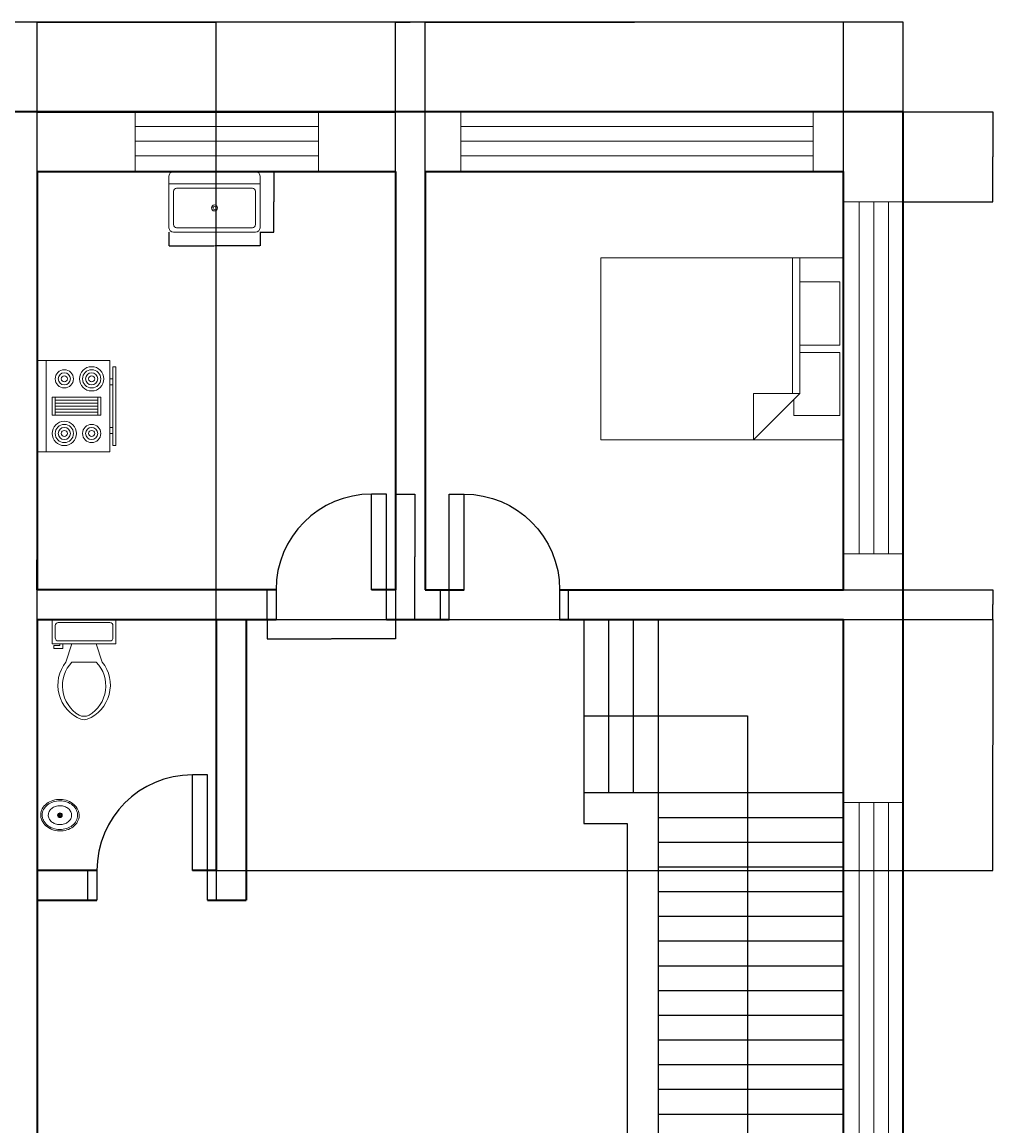
# Model space of a CAD drawing. Units: millimetres. Extents: x 726 to 37095, y -1634 to 13537.
# Tile 2 of 4: x 9102 to 17228, y 4296 to 13535. Entities that reach past the tile are written whole.
import ezdxf

# ---------------------------------------------------------------- set-up
doc = ezdxf.new("R2010")
doc.units = ezdxf.units.MM
for name, color, linetype, lineweight in [('A-ANNO-DIMS', 2, 'Continuous', 18), ('A-DOOR', 3, 'Continuous', 25), ('A-EQPM', 8, 'Continuous', 18), ('A-FLOR-FIXT', 9, 'Continuous', 18), ('A-FLOR-STRS', 5, 'Continuous', 25), ('A-FURN', 8, 'Continuous', 18), ('A-GLAZ', 4, 'Continuous', 18), ('A-WALL', 7, 'Continuous', 35)]:
    doc.layers.add(name, color=color, linetype=linetype, lineweight=lineweight)
doc.styles.get("Standard").update_dxf_attribs({"font": 'arial.ttf'})
doc.dimstyles.get("Standard").update_dxf_attribs({"dimtxt": 0.18, "dimasz": 0.18, "dimexe": 0.18, "dimexo": 0.0625, "dimgap": 0.09, "dimtad": 0, "dimtih": 1, "dimtoh": 1, "dimdec": 4, "dimzin": 0, "dimdsep": 46, "dimtxsty": 'Standard', "dimcen": 0.09, "dimadec": 0, "dimazin": 0, "dimtfac": 1, "dimtdec": 4, "dimtofl": 0, "dimtmove": 0, "dimatfit": 3, "dimfxl": 1, "dimtolj": 1, "dimtzin": 0, "dimarcsym": 0})

# ---------------------------------------------------------------- blocks, each defined once
blk = doc.blocks.new('Bed - Queen')
for p, q in [((0, -80.00003000000002), (0, 0)), ((0, 0), (59.99998999999999, 0)), ((59.99998999999999, 0), (59.99998999999999, -80.00003000000002)), ((7.99999, -1.200000000000017), (28.79998, -1.200000000000017)), ((7.99999, -14.4), (7.99999, -1.200000000000017)), ((28.79998, -1.200000000000017), (28.79998, -14.4)), ((31.19999, -1.200000000000017), (51.99999000000001, -1.200000000000017)), ((31.19999, -14.4), (31.19999, -1.200000000000017)), ((51.99999000000001, -1.200000000000017), (51.99999000000001, -16.4)), ((0, -14.4), (44.79999999999999, -14.4)), ((59.99998999999999, -29.60000000000001), (44.79999999999999, -14.4)), ((44.79999999999999, -14.4), (44.79999999999999, -29.60000000000001)), ((44.79999999999999, -16.80000000000001), (0, -16.80000000000001)), ((51.99999000000001, -16.4), (46.79936, -16.4)), ((44.79999999999999, -29.60000000000001), (59.99998999999999, -29.60000000000001)), ((59.99998999999999, -80.00003000000002), (0, -80.00003000000002))]:
    blk.add_line(p, q)
blk = doc.blocks.new('Toilet - top')
for p, q in [((9.5, -6), (9.5, -2)), ((-10, -8.5), (-8, -8.5)), ((-10, -9.5), (-10, -8.5)), ((-7, -9.5), (-10, -9.5)), ((-8, -8.5), (-8, -8)), ((-7, -8), (-7, -9.5)), ((-4, -8), (-6, -14)), ((4, -8), (6, -14)), ((4, -14), (-4, -14))]:
    blk.add_line(p, q)
blk.add_lwpolyline([(10.5, -8), (10.5, 0), (-10.5, 0), (-10.5, -8)], close=True)
for points in [[(-9.5, -2), (-9.5, -6)], [(8.5, -1), (-8.5, -1)], [(-8.5, -7), (8.5, -7)]]:
    blk.add_lwpolyline(points)
for centre, radius, start, end in [((-8.625, -1.875), 0.8838834999999999, 81.86989999999999, 188.1301), ((8.625, -1.875), 0.8838834999999999, 351.8699, 98.13009999999998), ((-8.625, -6.125), 0.8838834999999999, 171.869898, 278.1301), ((8.625, -6.125), 0.8838834999999999, 261.8699, 8.130099999999993), ((3.519562435188956, -21.58049502388982), 12.16902005083646, 141.4691096810948, 247.9714346835576), ((4.199957580658807, -21.81740929088453), 11.3291791325804, 136.3677254423718, 238.946823937405), ((-3.519499936778316, -21.58047137067522), 12.16903423757823, 292.0284332733152, 38.53070636800453), ((-4.199890672038477, -21.81738596564128), 11.32918622148567, 301.0530065773863, 43.63209216694732), ((2.09660981727e-05, -27.87646475467881), 4, 245.7318247449371, 294.2681740488959), ((2.09415214183e-05, -28.99996806116075), 4, 254.8605283244437, 285.1394707718433)]:
    blk.add_arc(centre, radius, start, end)
blk = doc.blocks.new('Sink - Oval top')
for p, q in [((-1, 0), (1, 0)), ((0, 1), (0, -1))]:
    blk.add_line(p, q)
for points in [[(-12.23371880354079, 0.3941914712607968, 0.1176342565883263), (-11.46456229543957, -3.361933235489118, 0.104469279667093), (-8.878748691070427, -6.803541973650567, 0.0900157896014849), (-5.082757700676665, -9.072309807490512, 0.0819199491592185), (-0.3227280122732736, -10.01585280257211, 0.0819199491592091), (4.488169920880977, -9.380701564817912, 0.0900157896014801), (8.422342359155778, -7.36101289847943, 0.1044692796670922), (11.22435122606941, -4.093009071543406, 0.1176342565883338), (12.23371880354091, -0.3941914712607968, 0.1176342565883057), (11.46456229543992, 3.361933235488777, 0.1044692796670849), (8.878748691070427, 6.803541973650567, 0.0900157896014884), (5.082757700676324, 9.072309807490681, 0.0819199491592058), (0.3227280122732736, 10.01585280257211, 0.081919949159207), (-4.488169920880864, 9.380701564817969, 0.0900157896014802), (-8.422342359155778, 7.36101289847943, 0.1044692796670951), (-11.22435122606919, 4.093009071543633, 0.1176342565883402)], [(-11.28627986850119, 0.1590597164737346, 0.1186217001864142), (-10.51590095791209, -3.253161772358112, 0.1046781721811095), (-8.071803350560115, -6.358618019863342, 0.0895620664691738), (-4.537699193222351, -8.366971929609804, 0.0811846988912177), (-0.1289739026695997, -9.15150355811437, 0.0811846988912276), (4.300109150126218, -8.491524865184601, 0.0895620664691798), (7.889406708212618, -6.583562428127606, 0.1046781721811044), (10.42004782883111, -3.548216131892445, 0.1186217001864013), (11.28627986850119, -0.1590597164736209, 0.1186217001863945), (10.51590095791221, 3.253161772357998, 0.1046781721811069), (8.071803350560115, 6.358618019863342, 0.0895620664691756), (4.537699193222124, 8.366971929609917, 0.081184698891216), (0.1289739026695997, 9.151503558114428, 0.0811846988912142), (-4.300109150125877, 8.491524865184829, 0.0895620664691747), (-7.889406708212618, 6.583562428127606, 0.1046781721811045), (-10.42004782883111, 3.548216131892445, 0.1186217001863946)], [(-7.420452389032902, 0.0829876781601797, 0.1182825673856775), (-6.907065465214486, -2.1674649380775, 0.1046074595377274), (-5.294791470712084, -4.209988192029413, 0.0897179636260996), (-2.966599981142508, -5.528122152688069, 0.0814360825277113), (-0.0675135187855176, -6.036810076758797, 0.0814360825277218), (2.84222437824053, -5.593085960977873, 0.0897179636261315), (5.199312936802016, -4.327350491993342, 0.1046074595376878), (6.85686365682659, -2.321395784920355, 0.1182825673856714), (7.420452389033016, -0.0829876781601797, 0.1182825673856961), (6.907065465214486, 2.167464938077614, 0.1046074595377135), (5.294791470712084, 4.209988192029413, 0.0897179636261265), (2.966599981142621, 5.528122152687842, 0.0814360825277426), (0.0675135187855176, 6.036810076758797, 0.0814360825277225), (-2.842224378240644, 5.593085960977873, 0.0897179636261212), (-5.199312936802016, 4.327350491993342, 0.1046074595377049), (-6.856863656826476, 2.321395784920355, 0.1182825673856712)]]:
    blk.add_lwpolyline(points, format="xyb", close=True)
for radius in [1.5, 1]:
    blk.add_circle((0, 0), radius)
blk = doc.blocks.new('Range-Oven - 30 in top')
for p, q in [((0, -3), (30, -3)), ((12, -6), (18, -6)), ((13, -19.999996), (13, -6)), ((14, -6), (14, -19.999996)), ((15, -19.999996), (15, -6)), ((16, -6), (16, -19.999996)), ((17, -19.999996), (17, -6)), ((18, -19.999996), (12, -19.999996)), ((6.000000000000003, -23.99999600000001), (6.000000000000003, -24.999996)), ((8.000000000000004, -24.999996), (8.000000000000004, -23.99999600000001)), ((22.00000000000001, -24.999996), (22.00000000000001, -23.99999600000001)), ((24, -23.99999600000001), (24, -24.999996))]:
    blk.add_line(p, q)
for points in [[(0, -23.99999600000001), (0, 0), (30, 0), (30, -23.99999600000001)], [(12, -20.999996), (12, -5), (18, -5), (18, -20.999996)], [(2.000000000000003, -25.999996), (2.000000000000003, -24.999996), (28.00000000000001, -24.999996), (28.00000000000001, -25.999996)]]:
    blk.add_lwpolyline(points, close=True)
for centre, radius in [((6.000000000000003, -9.0000002), 4), ((6.000000000000003, -9.0000002), 3), ((6.000000000000003, -9.0000002), 2), ((24, -9.0000002), 3), ((24, -9.0000002), 2), ((6.000000000000003, -9.0000002), 1), ((24, -9.0000002), 1), ((24, -18), 4), ((6.000000000000003, -18), 3), ((6.000000000000003, -18), 2), ((6.000000000000003, -18), 1), ((24, -18), 3), ((24, -18), 2), ((24, -18), 1)]:
    blk.add_circle(centre, radius)
blk = doc.blocks.new('Sink-single - 30 in top')
blk.add_line((-15, -3.999996000000001), (15, -3.999996000000001))
for points in [[(-13.5, 0), (13.5, 0)], [(-15, -18.499996), (-15, -1.500000000000001)], [(15, -1.500000000000001), (15, -18.499996)], [(-13.5, -17.499996), (-13.5, -6.499996000000001)], [(-12.5, -5.499996000000001), (12.5, -5.499996000000001)], [(13.5, -6.499996000000001), (13.5, -17.499996)], [(13.5, -19.999996), (-13.5, -19.999996)], [(12.5, -18.499996), (-12.5, -18.499996)]]:
    blk.add_lwpolyline(points)
for radius in [1, 0.5]:
    blk.add_circle((0, -11.999996), radius)
for centre, radius, start, end in [((-13.5, -1.500000000000001), 1.5, 90, 180), ((13.5, -1.500000000000001), 1.5, 0, 90), ((-12.5, -6.499996000000001), 1, 90, 180), ((12.5, -6.499996000000001), 1, 0, 90), ((-12.5, -17.499996), 1, 180, 270), ((12.5, -17.499996), 1, 270, 0), ((-13.5, -18.499996), 1.5, 180, 270), ((13.5, -18.499996), 1.5, 270, 0)]:
    blk.add_arc(centre, radius, start, end)
blk = doc.blocks.new('Window - Wood Frame 36 in. Wide plan')
for p, q in [((0, 6), (0, 0)), ((36, 6), (36, 0)), ((0, 4.5), (36, 4.5)), ((0, 3), (36, 3)), ((0, 1.5), (36, 1.5))]:
    blk.add_line(p, q)
blk = doc.blocks.new('DOOR-SWING-800')
for p, q in [((999.1999999999979, 1050), (874.1999999999979, 1050)), ((874.1999999999979, 250), (874.1999999999979, 1050)), ((999.1999999999979, 250), (999.1999999999979, 1050)), ((9.095e-13, 250), (74.199999999998, 250)), ((9.095e-13, 0), (9.095e-13, 250)), ((74.199999999998, 250), (74.199999999998, 0)), ((874.1999999999979, 250), (999.1999999999979, 250)), ((999.1999999999979, 250), (1073.400000000002, 250)), ((999.1999999999979, 0), (999.1999999999979, 250)), ((1073.400000000002, 250), (1073.400000000002, 0)), ((74.199999999998, 0), (9.095e-13, 0)), ((1073.400000000002, 0), (999.1999999999979, 0))]:
    blk.add_line(p, q)
blk.add_arc((874.1999999999979, 250), 800, 90, 180)
blk = doc.blocks.new('STAIR-QUARTER-TURN')
for p, q in [((1551.94660387568, 5000.000000000002), (1551.94660387568, 3551.516503049365)), ((1758.872817725773, 5000.000000000002), (1758.872817725773, 3551.516503049365)), ((1965.799031575862, 5000.000000000002), (1965.799031575862, 3551.516503049365)), ((2172.725245425954, 5000.000000000002), (2172.725245425954, 3551.516503049365)), ((2172.725245425954, 4193.579423830473), (803.743340616409, 4193.579423830471)), ((803.743340616409, 4193.579423830471), (803.743340616409, 330.5564002077117)), ((2172.725245425954, 3551.516503049366), (0, 3551.516503049365)), ((1551.94660387568, 3551.516503049365), (1551.94660387568, 3344.590289199272)), ((2172.725245425954, 3551.516503049365), (2172.725245425954, 3292.858735736751)), ((1551.94660387568, 3344.590289199272), (0, 3344.590289199273)), ((1551.94660387568, 3344.590289199272), (1551.94660387568, 861.4757229981805)), ((2172.725245425954, 3292.858735736751), (1810.604371188295, 3292.858735736751)), ((1810.604371188295, 3292.85873573675), (1810.604371188295, 602.8179556856148)), ((1551.94660387568, 3137.664075349182), (0, 3137.664075349182)), ((1551.94660387568, 2930.73786149909), (0, 2930.737861499091)), ((1551.94660387568, 2723.811647649), (0, 2723.811647649001)), ((1551.94660387568, 2516.885433798908), (0, 2516.885433798909)), ((1551.94660387568, 2309.959219948817), (0, 2309.959219948818)), ((1551.94660387568, 2103.033006098726), (0, 2103.033006098727)), ((1551.94660387568, 1896.106792248635), (0, 1896.106792248635)), ((1551.94660387568, 1689.180578398543), (0, 1689.180578398544)), ((1551.94660387568, 1482.254364548453), (0, 1482.254364548454)), ((1551.94660387568, 1275.328150698362), (0, 1275.328150698363)), ((1551.94660387568, 1068.40193684827), (0, 1068.401936848271)), ((1551.94660387568, 861.4757229981795), (0, 861.4757229981805)), ((1551.94660387568, 861.4757229981805), (1551.946603875687, 602.8179556856074)), ((1810.604371188295, 602.8179556856148), (1551.946603875687, 602.8179556855675)), ((803.743340616409, 330.5564002077117), (545.0855733037969, 330.5564002077117)), ((545.0855733037969, 330.5564002077117), (803.743340616409, 4.547e-13)), ((803.743340616409, 330.5564002077117), (1062.401107929021, 330.5564002077108)), ((803.743340616409, 4.547e-13), (1062.401107929021, 330.5564002077117))]:
    blk.add_line(p, q)
blk = doc.blocks.new('WIN-1535')
for p, q in [((0, 1.819e-12), (0, 500.0000000000036)), ((1534.861597237876, 1.819e-12), (1534.861597237876, 500.0000000000036)), ((-9.095e-13, 377.1532172399693), (1534.861597237876, 377.1532172399693)), ((-9.095e-13, 254.306434479935), (1534.861597237876, 254.306434479935)), ((-9.095e-13, 131.459651719897), (1534.861597237876, 131.4596517198988))]:
    blk.add_line(p, q)
blk = doc.blocks.new('*D19')
at = {"layer": 'A-ANNO-DIMS', "color": 0, "lineweight": -2, "transparency": 16777216}
for p, q in [((11153.90984586529, 8533.823368122881), (11153.90984586529, 8372.69586812288)), ((12227.30984586529, 8533.823368122881), (12227.30984586529, 8372.69586812288)), ((11154.08984586529, 8372.87586812288), (11688.87958665656, 8372.87586812288)), ((12227.12984586529, 8372.87586812288), (11692.34010507402, 8372.87586812288))]:
    blk.add_line(p, q, dxfattribs=at)
at = {"layer": 'A-ANNO-DIMS', "color": 0, "transparency": 16777216}
for points in [[(11154.08984586529, 8372.905868122883), (11154.08984586529, 8372.84586812288), (11153.90984586529, 8372.87586812288)], [(12227.12984586529, 8372.905868122883), (12227.12984586529, 8372.84586812288), (12227.30984586529, 8372.87586812288)]]:
    blk.add_solid(points, dxfattribs=at)
at = {"layer": 'Defpoints', "color": 0, "transparency": 16777216}
for p in [(11153.90984586529, 8533.885868122881), (12227.30984586529, 8533.885868122881), (12227.30984586529, 8372.87586812288)]:
    blk.add_point(p, dxfattribs=at)
at = {"layer": 'A-ANNO-DIMS', "color": 0, "transparency": 16777216, "insert": (11690.60984586529, 8372.87586812288), "char_height": 0.18, "attachment_point": 5}
blk.add_mtext('\\A1;INTERNAL DOOR 1073 TYP.', dxfattribs=at)
blk = doc.blocks.new('*D20')
at = {"layer": 'A-ANNO-DIMS', "color": 0, "lineweight": -2, "transparency": 16777216}
for p, q in [((12227.37234586529, 9583.885868122881), (12388.4998458653, 9583.885868122887)), ((12388.3198458653, 9583.705868122885), (12388.3198458653, 9059.067771260678)), ((12388.3198458653, 8534.065868122887), (12388.3198458653, 9058.703964985098)), ((12227.37234586529, 8533.885868122885), (12388.4998458653, 8533.885868122887))]:
    blk.add_line(p, q, dxfattribs=at)
at = {"layer": 'A-ANNO-DIMS', "color": 0, "transparency": 16777216}
for points in [[(12388.2898458653, 9583.705868122885), (12388.3498458653, 9583.705868122885), (12388.3198458653, 9583.885868122887)], [(12388.2898458653, 8534.065868122887), (12388.3498458653, 8534.065868122887), (12388.3198458653, 8533.885868122887)]]:
    blk.add_solid(points, dxfattribs=at)
at = {"layer": 'Defpoints', "color": 0, "transparency": 16777216}
for p in [(12227.30984586529, 9583.885868122881), (12388.3198458653, 9583.885868122887), (12227.30984586529, 8533.885868122885)]:
    blk.add_point(p, dxfattribs=at)
at = {"layer": 'A-ANNO-DIMS', "color": 0, "transparency": 16777216, "insert": (12388.3198458653, 9058.885868122881), "char_height": 0.18, "attachment_point": 5}
blk.add_mtext('\\A1;1050 TYP.', dxfattribs=at)
blk = doc.blocks.new('*D39')
at = {"layer": 'A-ANNO-DIMS', "color": 0, "lineweight": -2, "transparency": 16777216}
for p, q in [((10331.90706066462, 11775.82346972288), (10331.90706066462, 11661.40596972288)), ((11093.90706066462, 11775.82346972288), (11093.90706066462, 11661.40596972288)), ((10332.08706066462, 11661.58596972288), (10711.39787239722, 11661.58596972288)), ((11093.72706066462, 11661.58596972288), (10714.41624893201, 11661.58596972288))]:
    blk.add_line(p, q, dxfattribs=at)
at = {"layer": 'A-ANNO-DIMS', "color": 0, "transparency": 16777216}
for points in [[(10332.08706066462, 11661.61596972288), (10332.08706066462, 11661.55596972288), (10331.90706066462, 11661.58596972288)], [(11093.72706066462, 11661.61596972288), (11093.72706066462, 11661.55596972288), (11093.90706066462, 11661.58596972288)]]:
    blk.add_solid(points, dxfattribs=at)
at = {"layer": 'Defpoints', "color": 0, "transparency": 16777216}
for p in [(10331.90706066462, 11775.88596972288), (11093.90706066462, 11775.88596972288), (11093.90706066462, 11661.58596972288)]:
    blk.add_point(p, dxfattribs=at)
at = {"layer": 'A-ANNO-DIMS', "color": 0, "transparency": 16777216, "insert": (10712.90706066462, 11661.58596972288), "char_height": 0.18, "attachment_point": 5}
blk.add_mtext('\\A1;KITCHEN SINK 762 TYP.', dxfattribs=at)
blk = doc.blocks.new('*D40')
at = {"layer": 'A-ANNO-DIMS', "color": 0, "lineweight": -2, "transparency": 16777216}
for p, q in [((11093.96956066462, 12283.88586812288), (11208.38706066463, 12283.88586812288)), ((11208.20706066463, 12283.70586812288), (11208.20706066463, 12030.06782206067)), ((11208.20706066463, 11776.06596972288), (11208.20706066463, 12029.70401578509)), ((11093.96956066462, 11775.88596972288), (11208.38706066463, 11775.88596972288))]:
    blk.add_line(p, q, dxfattribs=at)
at = {"layer": 'A-ANNO-DIMS', "color": 0, "transparency": 16777216}
for points in [[(11208.17706066462, 12283.70586812288), (11208.23706066462, 12283.70586812288), (11208.20706066463, 12283.88586812288)], [(11208.17706066462, 11776.06596972288), (11208.23706066462, 11776.06596972288), (11208.20706066463, 11775.88596972288)]]:
    blk.add_solid(points, dxfattribs=at)
at = {"layer": 'Defpoints', "color": 0, "transparency": 16777216}
for p in [(11093.90706066462, 12283.88586812288), (11208.20706066463, 12283.88586812288), (11093.90706066462, 11775.88596972288)]:
    blk.add_point(p, dxfattribs=at)
at = {"layer": 'A-ANNO-DIMS', "color": 0, "transparency": 16777216, "insert": (11208.20706066463, 12029.88591892288), "char_height": 0.18, "attachment_point": 5}
blk.add_mtext('\\A1;508 TYP.', dxfattribs=at)
blk = doc.blocks.new('*D43')
at = {"layer": 'A-ANNO-DIMS', "color": 0, "lineweight": -2, "transparency": 16777216}
for p, q in [((1477.309846, 12783.948368), (1477.309846, 13534.815868)), ((1477.489846, 13534.635868), (8976.889927855387, 13534.635868)), ((16477.129846, 13534.635868), (8977.72976414461, 13534.635868)), ((16477.309846, 12783.948368), (16477.309846, 13534.815868))]:
    blk.add_line(p, q, dxfattribs=at)
at = {"layer": 'A-ANNO-DIMS', "color": 0, "transparency": 16777216}
for points in [[(1477.489846, 13534.665868), (1477.489846, 13534.605868), (1477.309846, 13534.635868)], [(16477.129846, 13534.665868), (16477.129846, 13534.605868), (16477.309846, 13534.635868)]]:
    blk.add_solid(points, dxfattribs=at)
at = {"layer": 'Defpoints', "color": 0, "transparency": 16777216}
for p in [(16477.309846, 13534.635868), (1477.309846, 12783.885868), (16477.309846, 12783.885868)]:
    blk.add_point(p, dxfattribs=at)
at = {"layer": 'A-ANNO-DIMS', "color": 0, "transparency": 16777216, "insert": (8977.309846, 13534.635868), "char_height": 0.18, "attachment_point": 5}
blk.add_mtext('\\A1;15000', dxfattribs=at)
blk = doc.blocks.new('*D48')
at = {"layer": 'A-ANNO-DIMS', "color": 0, "lineweight": -2, "transparency": 16777216}
for p, q in [((8727.309846, 12283.948368), (8727.309846, 13534.815868)), ((8727.489846, 13534.635868), (8977.021305754433, 13534.635868)), ((9227.129846, 13534.635868), (8977.598386245567, 13534.635868)), ((9227.309846, 12283.948368), (9227.309846, 13534.815868))]:
    blk.add_line(p, q, dxfattribs=at)
at = {"layer": 'A-ANNO-DIMS', "color": 0, "transparency": 16777216}
for points in [[(8727.489846, 13534.665868), (8727.489846, 13534.605868), (8727.309846, 13534.635868)], [(9227.129846, 13534.665868), (9227.129846, 13534.605868), (9227.309846, 13534.635868)]]:
    blk.add_solid(points, dxfattribs=at)
at = {"layer": 'Defpoints', "color": 0, "transparency": 16777216}
for p in [(9227.309846, 13534.635868), (8727.309846, 12283.885868), (9227.309846, 12283.885868)]:
    blk.add_point(p, dxfattribs=at)
at = {"layer": 'A-ANNO-DIMS', "color": 0, "transparency": 16777216, "insert": (8977.309846, 13534.635868), "char_height": 0.18, "attachment_point": 5}
blk.add_mtext('\\A1;500', dxfattribs=at)
blk = doc.blocks.new('*D49')
at = {"layer": 'A-ANNO-DIMS', "color": 0, "lineweight": -2, "transparency": 16777216}
for p, q in [((9227.309846, 12283.948368), (9227.309846, 13534.815868)), ((9227.489846, 13534.635868), (10726.95144218008, 13534.635868)), ((12227.129846, 13534.635868), (10727.66824981992, 13534.635868)), ((12227.309846, 12283.948368), (12227.309846, 13534.815868))]:
    blk.add_line(p, q, dxfattribs=at)
at = {"layer": 'A-ANNO-DIMS', "color": 0, "transparency": 16777216}
for points in [[(9227.489846, 13534.665868), (9227.489846, 13534.605868), (9227.309846, 13534.635868)], [(12227.129846, 13534.665868), (12227.129846, 13534.605868), (12227.309846, 13534.635868)]]:
    blk.add_solid(points, dxfattribs=at)
at = {"layer": 'Defpoints', "color": 0, "transparency": 16777216}
for p in [(12227.309846, 13534.635868), (9227.309846, 12283.885868), (12227.309846, 12283.885868)]:
    blk.add_point(p, dxfattribs=at)
at = {"layer": 'A-ANNO-DIMS', "color": 0, "transparency": 16777216, "insert": (10727.309846, 13534.635868), "char_height": 0.18, "attachment_point": 5}
blk.add_mtext('\\A1;3000', dxfattribs=at)
blk = doc.blocks.new('*D50')
at = {"layer": 'A-ANNO-DIMS', "color": 0, "lineweight": -2, "transparency": 16777216}
for p, q in [((12227.309846, 12283.948368), (12227.309846, 13534.815868)), ((12227.489846, 13534.635868), (12352.01977096589, 13534.635868)), ((12477.129846, 13534.635868), (12352.59992103411, 13534.635868)), ((12477.309846, 12283.948368), (12477.309846, 13534.815868))]:
    blk.add_line(p, q, dxfattribs=at)
at = {"layer": 'A-ANNO-DIMS', "color": 0, "transparency": 16777216}
for points in [[(12227.489846, 13534.665868), (12227.489846, 13534.605868), (12227.309846, 13534.635868)], [(12477.129846, 13534.665868), (12477.129846, 13534.605868), (12477.309846, 13534.635868)]]:
    blk.add_solid(points, dxfattribs=at)
at = {"layer": 'Defpoints', "color": 0, "transparency": 16777216}
for p in [(12477.309846, 13534.635868), (12227.309846, 12283.885868), (12477.309846, 12283.885868)]:
    blk.add_point(p, dxfattribs=at)
at = {"layer": 'A-ANNO-DIMS', "color": 0, "transparency": 16777216, "insert": (12352.309846, 13534.635868), "char_height": 0.18, "attachment_point": 5}
blk.add_mtext('\\A1;250', dxfattribs=at)
blk = doc.blocks.new('*D51')
at = {"layer": 'A-ANNO-DIMS', "color": 0, "lineweight": -2, "transparency": 16777216}
for p, q in [((12477.309846, 12283.948368), (12477.309846, 13534.815868)), ((12477.489846, 13534.635868), (14226.95144218008, 13534.635868)), ((15977.129846, 13534.635868), (14227.66824981992, 13534.635868)), ((15977.309846, 12283.948368), (15977.309846, 13534.815868))]:
    blk.add_line(p, q, dxfattribs=at)
at = {"layer": 'A-ANNO-DIMS', "color": 0, "transparency": 16777216}
for points in [[(12477.489846, 13534.665868), (12477.489846, 13534.605868), (12477.309846, 13534.635868)], [(15977.129846, 13534.665868), (15977.129846, 13534.605868), (15977.309846, 13534.635868)]]:
    blk.add_solid(points, dxfattribs=at)
at = {"layer": 'Defpoints', "color": 0, "transparency": 16777216}
for p in [(15977.309846, 13534.635868), (12477.309846, 12283.885868), (15977.309846, 12283.885868)]:
    blk.add_point(p, dxfattribs=at)
at = {"layer": 'A-ANNO-DIMS', "color": 0, "transparency": 16777216, "insert": (14227.309846, 13534.635868), "char_height": 0.18, "attachment_point": 5}
blk.add_mtext('\\A1;3500', dxfattribs=at)
blk = doc.blocks.new('*D54')
at = {"layer": 'A-ANNO-DIMS', "color": 0, "lineweight": -2, "transparency": 16777216}
for p, q in [((15977.372346, 8783.885868000005), (17228.23984600001, 8783.885868000005)), ((17228.05984600001, 8783.705868000003), (17228.05984600001, 8659.067771137792)), ((17228.05984600001, 8534.065868000003), (17228.05984600001, 8658.703964862214)), ((15977.372346, 8533.885868000005), (17228.23984600001, 8533.885868000005))]:
    blk.add_line(p, q, dxfattribs=at)
at = {"layer": 'A-ANNO-DIMS', "color": 0, "transparency": 16777216}
for points in [[(17228.02984600001, 8783.705868000003), (17228.08984600001, 8783.705868000003), (17228.05984600001, 8783.885868000005)], [(17228.02984600001, 8534.065868000003), (17228.08984600001, 8534.065868000003), (17228.05984600001, 8533.885868000005)]]:
    blk.add_solid(points, dxfattribs=at)
at = {"layer": 'Defpoints', "color": 0, "transparency": 16777216}
for p in [(15977.309846, 8783.885868000005), (15977.309846, 8533.885868000005), (17228.05984600001, 8533.885868000005)]:
    blk.add_point(p, dxfattribs=at)
at = {"layer": 'A-ANNO-DIMS', "color": 0, "transparency": 16777216, "insert": (17228.05984600001, 8658.885867999996), "char_height": 0.18, "attachment_point": 5}
blk.add_mtext('\\A1;250', dxfattribs=at)
blk = doc.blocks.new('*D55')
at = {"layer": 'A-ANNO-DIMS', "color": 0, "lineweight": -2, "transparency": 16777216}
for p, q in [((10727.372346, 8533.885868000005), (17228.23984600001, 8533.885868000005)), ((17228.05984600001, 8533.705868000003), (17228.05984600001, 7484.067771137794)), ((17228.05984600001, 6434.065868000004), (17228.05984600001, 7483.703964862215)), ((10727.372346, 6433.885868000004), (17228.23984600001, 6433.885868000004))]:
    blk.add_line(p, q, dxfattribs=at)
at = {"layer": 'A-ANNO-DIMS', "color": 0, "transparency": 16777216}
for points in [[(17228.02984600001, 8533.705868000003), (17228.08984600001, 8533.705868000003), (17228.05984600001, 8533.885868000005)], [(17228.02984600001, 6434.065868000004), (17228.08984600001, 6434.065868000004), (17228.05984600001, 6433.885868000004)]]:
    blk.add_solid(points, dxfattribs=at)
at = {"layer": 'Defpoints', "color": 0, "transparency": 16777216}
for p in [(10727.309846, 8533.885868000005), (10727.309846, 6433.885868000004), (17228.05984600001, 6433.885868000004)]:
    blk.add_point(p, dxfattribs=at)
at = {"layer": 'A-ANNO-DIMS', "color": 0, "transparency": 16777216, "insert": (17228.05984600001, 7483.885867999998), "char_height": 0.18, "attachment_point": 5}
blk.add_mtext('\\A1;2100', dxfattribs=at)
blk = doc.blocks.new('*D56')
at = {"layer": 'A-ANNO-DIMS', "color": 0, "lineweight": -2, "transparency": 16777216}
for p, q in [((9227.309846, 6433.948368), (9227.309846, 13534.815868)), ((9227.489846, 13534.635868), (9976.959852821283, 13534.635868)), ((10727.129846, 13534.635868), (9977.659839178717, 13534.635868)), ((10727.309846, 6433.948368), (10727.309846, 13534.815868))]:
    blk.add_line(p, q, dxfattribs=at)
at = {"layer": 'A-ANNO-DIMS', "color": 0, "transparency": 16777216}
for points in [[(9227.489846, 13534.665868), (9227.489846, 13534.605868), (9227.309846, 13534.635868)], [(10727.129846, 13534.665868), (10727.129846, 13534.605868), (10727.309846, 13534.635868)]]:
    blk.add_solid(points, dxfattribs=at)
at = {"layer": 'Defpoints', "color": 0, "transparency": 16777216}
for p in [(9227.309846, 13534.635868), (9227.309846, 6433.885868), (10727.309846, 6433.885868)]:
    blk.add_point(p, dxfattribs=at)
at = {"layer": 'A-ANNO-DIMS', "color": 0, "transparency": 16777216, "insert": (9977.309846, 13534.635868), "char_height": 0.18, "attachment_point": 5}
blk.add_mtext('\\A1;1500', dxfattribs=at)
blk = doc.blocks.new('*D62')
at = {"layer": 'A-ANNO-DIMS', "color": 0, "lineweight": -2, "transparency": 16777216}
for p, q in [((16477.372346, 12783.885868), (17228.23984600001, 12783.885868)), ((17228.05984600001, 12783.705868), (17228.05984600001, 12407.80085563779)), ((17228.05984600001, 12031.532037), (17228.05984600001, 12407.43704936221)), ((16477.372346, 12031.352037), (17228.23984600001, 12031.352037))]:
    blk.add_line(p, q, dxfattribs=at)
at = {"layer": 'A-ANNO-DIMS', "color": 0, "transparency": 16777216}
for points in [[(17228.02984600001, 12783.705868), (17228.08984600001, 12783.705868), (17228.05984600001, 12783.885868)], [(17228.02984600001, 12031.532037), (17228.08984600001, 12031.532037), (17228.05984600001, 12031.352037)]]:
    blk.add_solid(points, dxfattribs=at)
at = {"layer": 'Defpoints', "color": 0, "transparency": 16777216}
for p in [(16477.309846, 12783.885868), (17228.05984600001, 12783.885868), (16477.309846, 12031.352037)]:
    blk.add_point(p, dxfattribs=at)
at = {"layer": 'A-ANNO-DIMS', "color": 0, "transparency": 16777216, "insert": (17228.05984600001, 12407.61895249999), "char_height": 0.18, "attachment_point": 5}
blk.add_mtext('\\A1;752.5', dxfattribs=at)

msp = doc.modelspace()

# ---------------------------------------------------------------- linework, layer by layer
at = {"layer": 'A-DOOR'}
for p, q in [((12153.10984586528, 8783.885868122885), (12028.10984586528, 8783.885868122885)), ((12602.30984586529, 8783.885868122885), (12602.30984586529, 8533.885868122885)), ((12676.50984586529, 8783.885868122885), (12801.50984586529, 8783.885868122885)), ((10653.10984586528, 6433.885868122885), (10528.10984586528, 6433.885868122885))]:
    msp.add_line(p, q, dxfattribs=at)
at = {"layer": 'A-FLOR-STRS'}
for p, q in [((13804.58460043933, 8533.885868122885), (13804.58460043933, 7085.402371172247)), ((13804.58460043933, 7085.402371172247), (13804.58460043933, 6826.744603859634))]:
    msp.add_line(p, q, dxfattribs=at)
at = {"layer": 'A-WALL'}
for p, q in [((16477.30984586529, 12783.88586812288), (1477.309845865288, 12783.88586812288)), ((9227.309845865288, 12783.88586812288), (12227.30984586529, 12783.88586812288)), ((15977.30984586529, 12783.88586812288), (12477.30984586529, 12783.88586812288)), ((16477.30984586529, 783.8858681228857), (16477.30984586529, 12783.88586812288)), ((9227.30984586529, 12283.88586812288), (9227.309845865288, 8783.885868122885)), ((9227.30984586529, 12283.88586812288), (12227.30984586528, 12283.88586812288)), ((12227.30984586529, 12283.88586812288), (12227.30984586529, 9283.885868122885)), ((12477.30984586529, 12283.88586812288), (12477.30984586529, 8783.885868122885)), ((12477.30984586529, 12283.88586812288), (15977.30984586529, 12283.88586812288)), ((15977.30984586529, 8783.885868122885), (15977.30984586529, 12283.88586812288)), ((12227.30984586529, 9283.885868122885), (12227.30984586529, 9033.885868122885)), ((9227.309845865288, 8783.885868122885), (9227.309845865288, 9033.885868122885)), ((12227.30984586529, 9033.885868122885), (12227.30984586529, 8783.885868122885)), ((11228.10984586528, 8783.885868122885), (9227.309845865288, 8783.885868122885)), ((12227.30984586528, 8783.885868122887), (12028.10984586528, 8783.885868122885)), ((12477.30984586529, 8783.885868122885), (12801.50984586529, 8783.885868122885)), ((13601.50984586529, 8783.885868122885), (15977.30984586529, 8783.885868122885)), ((9227.30984586529, 8533.885868122885), (11228.10984586528, 8533.885868122885)), ((9227.30984586529, 8533.885868122885), (9227.30984586529, 1283.885868122886)), ((10727.30984586529, 8533.885868122885), (10727.30984586529, 6433.885868122885)), ((10977.30984586529, 8533.885868122885), (10977.30984586529, 6184.561644066505)), ((12153.10984586528, 8533.885868122885), (12676.50984586529, 8533.885868122885)), ((13601.50984586529, 8533.885868122885), (15977.30984586529, 8533.885868122885)), ((13804.58460043933, 8533.885868122885), (15977.30984586529, 8533.885868122885)), ((15977.30984586529, 1283.885868122886), (15977.30984586529, 8533.885868122885)), ((15977.30984586529, 4395.361591121064), (15977.30984586529, 8533.885868122883)), ((9227.30984586529, 6933.885868122885), (9227.30984586529, 4433.885868122884)), ((9728.109845865285, 6433.885868122885), (9227.30984586529, 6433.885868122885)), ((10727.30984586529, 6433.885868122885), (10528.10984586528, 6433.885868122885)), ((9227.30984586529, 6184.561644066505), (9728.109845865285, 6184.561644066505)), ((10653.10984586528, 6184.561644066505), (10977.30984586529, 6184.561644066505))]:
    msp.add_line(p, q, dxfattribs=at)

# ---------------------------------------------------------------- block references
at = {"layer": 'A-DOOR'}
for p in [(11153.90984586529, 8533.885868122881), (9653.90984586529, 6183.885868122882)]:
    msp.add_blockref('DOOR-SWING-800', p, dxfattribs=at)
at = {"layer": 'A-DOOR', "extrusion": (0, 0, -1), "zscale": -1}
msp.add_blockref('DOOR-SWING-800', (-13675.70984586529, 8533.885868122885), dxfattribs=at)
at = {"layer": 'A-EQPM', "xscale": 25.4, "yscale": 25.4, "zscale": 25.4, "rotation": 89.99999999999999}
msp.add_blockref('Range-Oven - 30 in top', (9227.30984586529, 9939.069495433216), dxfattribs=at)
at = {"layer": 'A-FLOR-FIXT'}
for name, p, xscale, yscale, zscale in [('Sink-single - 30 in top', (10712.90706066462, 12283.88586812288), 25.4, 25.4, 25.4), ('Toilet - top', (9621.414881966515, 8533.885868122885), 25.4, 25.4, 25.4), ('Sink - Oval top', (9419.204158184584, 6896.535276851754), 13.14744327818227, 13.14744327818227, 13.14744327818227)]:
    msp.add_blockref(name, p, dxfattribs=dict(at, xscale=xscale, yscale=yscale, zscale=zscale))
at = {"layer": 'A-FLOR-STRS', "extrusion": (0, 0, -1), "zscale": -1}
msp.add_blockref('STAIR-QUARTER-TURN', (-15977.30984586528, 3533.885868122882), dxfattribs=at)
at = {"layer": 'A-FURN', "xscale": 25.4, "yscale": 25.4, "zscale": 25.4, "rotation": 270}
msp.add_blockref('Bed - Queen', (15977.30984586529, 11562.56026255546), dxfattribs=at)
at = {"layer": 'A-GLAZ'}
msp.add_blockref('WIN-1535', (10049.2141855713, 12283.88586812288), dxfattribs=at)
at = {"layer": 'A-GLAZ', "xscale": 81.8978551733564, "yscale": 81.8978551733564, "zscale": 81.8978551733564}
msp.add_blockref('Window - Wood Frame 36 in. Wide plan', (12774.18160980101, 12292.49873708274), dxfattribs=at)
at = {"layer": 'A-GLAZ', "xscale": 81.8978551733564, "yscale": 81.8978551733564, "zscale": 81.8978551733564, "rotation": 270}
for p in [(15985.92271482515, 12031.35203741656), (15985.92271482514, 7003.139441062607)]:
    msp.add_blockref('Window - Wood Frame 36 in. Wide plan', p, dxfattribs=at)

# ---------------------------------------------------------------- dimensions: what is measured, and where the dimension line sits
at = {"layer": 'A-ANNO-DIMS'}
for base, p1, p2, picture, middle in [((16477.309846, 13534.635868), (1477.309846, 12783.885868), (16477.309846, 12783.885868), '*D43', (8977.309846, 13534.635868)), ((9227.309846, 13534.635868), (8727.309846, 12283.885868), (9227.309846, 12283.885868), '*D48', (8977.309846, 13534.635868)), ((12227.309846, 13534.635868), (9227.309846, 12283.885868), (12227.309846, 12283.885868), '*D49', (10727.309846, 13534.635868)), ((9227.309846, 13534.635868), (10727.309846, 6433.885868), (9227.309846, 6433.885868), '*D56', (9977.309846, 13534.635868)), ((12477.309846, 13534.635868), (12227.309846, 12283.885868), (12477.309846, 12283.885868), '*D50', (12352.309846, 13534.635868)), ((15977.309846, 13534.635868), (12477.309846, 12283.885868), (15977.309846, 12283.885868), '*D51', (14227.309846, 13534.635868))]:
    dim = msp.add_linear_dim(base=base, p1=p1, p2=p2, dimstyle='Standard', override={"dimdec": 0, "dimlfac": 1, "dimrnd": 0, "dimzin": 0, "dimdsep": 46, "dimlunit": 2}, dxfattribs=at)
    dim.commit()
    dim.dimension.update_dxf_attribs({"geometry": picture, "text_midpoint": middle})
for base, p1, p2, override, picture, middle in [((17228.05984600001, 12783.885868), (16477.309846, 12031.352037), (16477.309846, 12783.885868), {"dimdec": 1, "dimlfac": 1, "dimrnd": 0, "dimzin": 0, "dimdsep": 46, "dimlunit": 2}, '*D62', (17228.05984600001, 12407.61895249999)), ((17228.05984600001, 8533.885868000005), (15977.309846, 8783.885868), (15977.309846, 8533.885868), {"dimdec": 0, "dimlfac": 1, "dimrnd": 0, "dimzin": 0, "dimdsep": 46, "dimlunit": 2}, '*D54', (17228.05984600001, 8658.885867999996)), ((17228.05984600001, 6433.885868000004), (10727.309846, 8533.885868), (10727.309846, 6433.885868), {"dimdec": 0, "dimlfac": 1, "dimrnd": 0, "dimzin": 0, "dimdsep": 46, "dimlunit": 2}, '*D55', (17228.05984600001, 7483.885867999998))]:
    dim = msp.add_linear_dim(base=base, p1=p1, p2=p2, angle=90, dimstyle='Standard', override=override, dxfattribs=at)
    dim.commit()
    dim.dimension.update_dxf_attribs({"geometry": picture, "text_midpoint": middle})
for base, p1, p2, picture, middle in [((11208.20706066463, 12283.88586812288), (11093.90706066462, 11775.88596972288), (11093.90706066462, 12283.88586812288), '*D40', (11208.20706066463, 12029.88591892288)), ((12388.3198458653, 9583.885868122887), (12227.30984586529, 8533.885868122881), (12227.30984586529, 9583.88586812288), '*D20', (12388.3198458653, 9058.885868122881))]:
    dim = msp.add_linear_dim(base=base, p1=p1, p2=p2, angle=90, text='<> TYP.', dimstyle='Standard', override={"dimdec": 0, "dimlfac": 1, "dimrnd": 0, "dimzin": 0, "dimdsep": 46, "dimlunit": 2}, dxfattribs=at)
    dim.commit()
    dim.dimension.update_dxf_attribs({"geometry": picture, "text_midpoint": middle})
for base, p1, p2, text, picture, middle in [((11093.90706066462, 11661.58596972288), (10331.90706066462, 11775.88596972288), (11093.90706066462, 11775.88596972288), 'KITCHEN SINK <> TYP.', '*D39', (10712.90706066462, 11661.58596972288)), ((12227.30984586529, 8372.87586812288), (11153.90984586529, 8533.885868122881), (12227.30984586529, 8533.885868122881), 'INTERNAL DOOR <> TYP.', '*D19', (11690.60984586529, 8372.87586812288))]:
    dim = msp.add_linear_dim(base=base, p1=p1, p2=p2, text=text, dimstyle='Standard', override={"dimdec": 0, "dimlfac": 1, "dimrnd": 0, "dimzin": 0, "dimdsep": 46, "dimlunit": 2}, dxfattribs=at)
    dim.commit()
    dim.dimension.update_dxf_attribs({"geometry": picture, "text_midpoint": middle})

doc.saveas('drawing.dxf')
